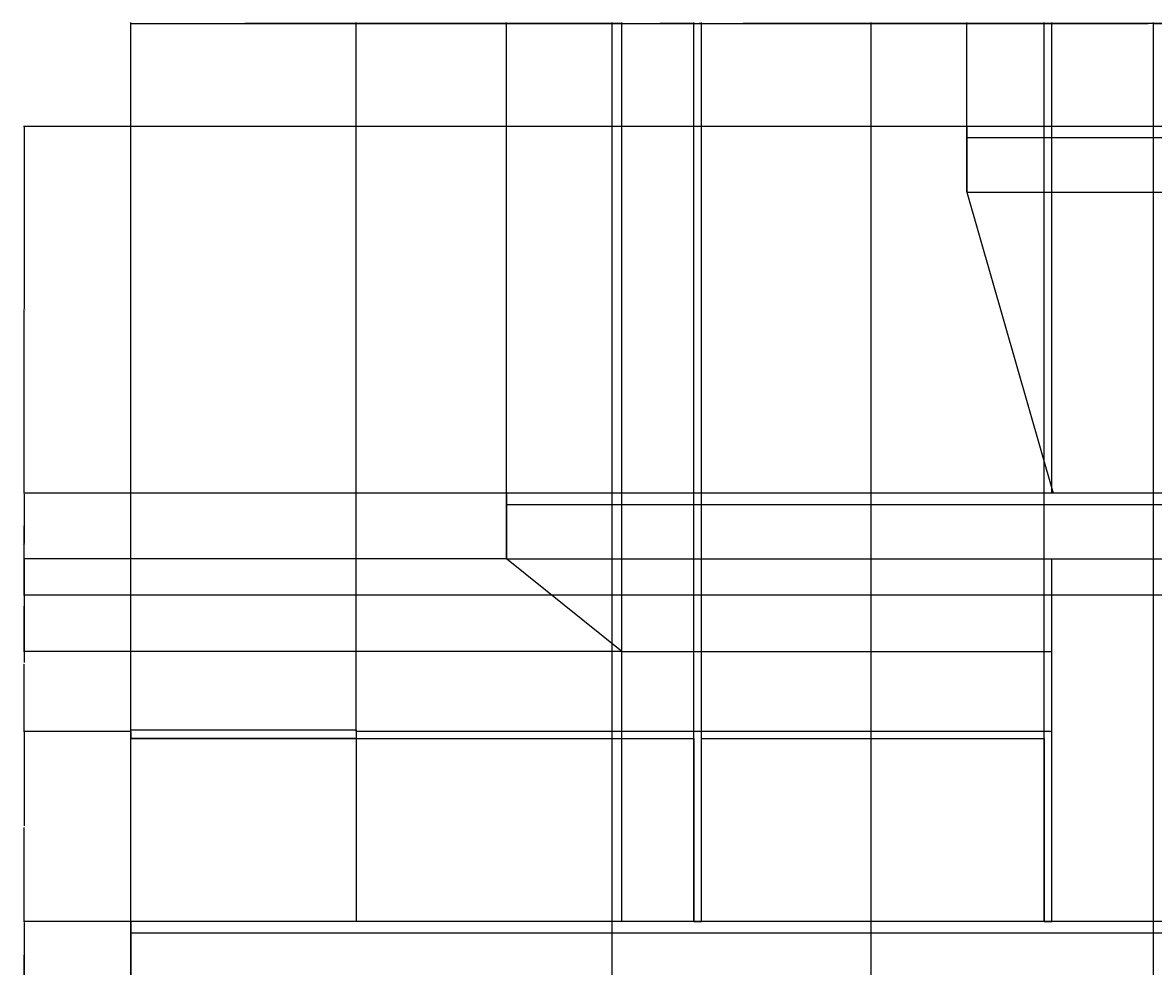
# Model space of a CAD drawing. Units: feet. Extents: x 2926 to 4178, y 965 to 1469.
# Tile 8 of 9: x 3641 to 3913, y 1241 to 1469. Entities that reach past the tile are written whole.
import ezdxf

# ---------------------------------------------------------------- set-up
doc = ezdxf.new("R2010")
doc.units = ezdxf.units.FT
doc.layers.add('A-ANNO-DIMS', color=2, linetype='Continuous', lineweight=18)
doc.layers.add('A-ELEV', color=7, linetype='Continuous', lineweight=25)
doc.styles.get("Standard").update_dxf_attribs({"font": 'arial.ttf'})
doc.dimstyles.get("Standard").update_dxf_attribs({"dimtxt": 0.18, "dimasz": 0.18, "dimexe": 0.18, "dimexo": 0.0625, "dimgap": 0.09, "dimtad": 0, "dimtih": 1, "dimtoh": 1, "dimdec": 1, "dimzin": 0, "dimdsep": 46, "dimlunit": 3, "dimtxsty": 'Standard', "dimcen": 0.09, "dimadec": 0, "dimazin": 0, "dimtfac": 1, "dimtdec": 1, "dimtofl": 0, "dimtmove": 0, "dimatfit": 3, "dimfxl": 1, "dimtolj": 1, "dimtzin": 0, "dimarcsym": 0})

# ---------------------------------------------------------------- blocks, each defined once
blk = doc.blocks.new('*D74')
at = {"layer": 'A-ANNO-DIMS', "color": 0, "lineweight": -2, "transparency": 16777216}
for p, q in [((3667.11, 1298.4), (3667.11, 1468.62)), ((3667.29, 1468.44), (3909.8, 1468.44)), ((4153.1, 1468.44), (3910.59, 1468.44)), ((4153.28, 1443.71), (4153.28, 1468.62))]:
    blk.add_line(p, q, dxfattribs=at)
at = {"layer": 'A-ANNO-DIMS', "color": 0, "transparency": 16777216}
for points in [[(3667.29, 1468.47), (3667.29, 1468.41), (3667.11, 1468.44)], [(4153.1, 1468.47), (4153.1, 1468.41), (4153.28, 1468.44)]]:
    blk.add_solid(points, dxfattribs=at)
at = {"layer": 'Defpoints', "color": 0, "transparency": 16777216}
for p in [(4153.28, 1468.44), (4153.28, 1443.64), (3667.11, 1298.33)]:
    blk.add_point(p, dxfattribs=at)
at = {"layer": 'A-ANNO-DIMS', "color": 0, "transparency": 16777216, "insert": (3910.2, 1468.44), "char_height": 0.18, "attachment_point": 5}
blk.add_mtext('\\A1;486.2', dxfattribs=at)
blk = doc.blocks.new('*D81')
at = {"layer": 'A-ANNO-DIMS', "color": 0, "lineweight": -2, "transparency": 16777216}
for p, q in [((3667.05, 1252.14), (3641.28, 1252.14)), ((3641.46, 1251.96), (3641.46, 1235.86)), ((3641.46, 1219.4), (3641.46, 1235.5)), ((3913.29, 1219.22), (3641.28, 1219.22))]:
    blk.add_line(p, q, dxfattribs=at)
at = {"layer": 'A-ANNO-DIMS', "color": 0, "transparency": 16777216}
for points in [[(3641.43, 1251.96), (3641.49, 1251.96), (3641.46, 1252.14)], [(3641.43, 1219.4), (3641.49, 1219.4), (3641.46, 1219.22)]]:
    blk.add_solid(points, dxfattribs=at)
at = {"layer": 'Defpoints', "color": 0, "transparency": 16777216}
for p in [(3641.46, 1252.14), (3667.11, 1252.14), (3913.35, 1219.22)]:
    blk.add_point(p, dxfattribs=at)
at = {"layer": 'A-ANNO-DIMS', "color": 0, "transparency": 16777216, "insert": (3641.46, 1235.68), "char_height": 0.18, "attachment_point": 5}
blk.add_mtext('\\A1;32.92', dxfattribs=at)
blk = doc.blocks.new('*D82')
at = {"layer": 'A-ANNO-DIMS', "color": 0, "lineweight": -2, "transparency": 16777216}
for p, q in [((3667.05, 1297.9), (3641.28, 1297.9)), ((3641.46, 1297.72), (3641.46, 1275.2)), ((3641.46, 1252.32), (3641.46, 1274.84)), ((3667.05, 1252.14), (3641.28, 1252.14))]:
    blk.add_line(p, q, dxfattribs=at)
at = {"layer": 'A-ANNO-DIMS', "color": 0, "transparency": 16777216}
for points in [[(3641.43, 1297.72), (3641.49, 1297.72), (3641.46, 1297.9)], [(3641.43, 1252.32), (3641.49, 1252.32), (3641.46, 1252.14)]]:
    blk.add_solid(points, dxfattribs=at)
at = {"layer": 'Defpoints', "color": 0, "transparency": 16777216}
for p in [(3641.46, 1297.9), (3667.11, 1297.9), (3667.11, 1252.14)]:
    blk.add_point(p, dxfattribs=at)
at = {"layer": 'A-ANNO-DIMS', "color": 0, "transparency": 16777216, "insert": (3641.46, 1275.02), "char_height": 0.18, "attachment_point": 5}
blk.add_mtext('\\A1;45.76', dxfattribs=at)
blk = doc.blocks.new('*D83')
at = {"layer": 'A-ANNO-DIMS', "color": 0, "lineweight": -2, "transparency": 16777216}
for p, q in [((4050.56, 1330.74), (3641.28, 1330.74)), ((3641.46, 1330.56), (3641.46, 1314.5)), ((3641.46, 1298.08), (3641.46, 1314.14)), ((3667.05, 1297.9), (3641.28, 1297.9))]:
    blk.add_line(p, q, dxfattribs=at)
at = {"layer": 'A-ANNO-DIMS', "color": 0, "transparency": 16777216}
for points in [[(3641.43, 1330.56), (3641.49, 1330.56), (3641.46, 1330.74)], [(3641.43, 1298.08), (3641.49, 1298.08), (3641.46, 1297.9)]]:
    blk.add_solid(points, dxfattribs=at)
at = {"layer": 'Defpoints', "color": 0, "transparency": 16777216}
for p in [(3641.46, 1330.74), (4050.62, 1330.74), (3667.11, 1297.9)]:
    blk.add_point(p, dxfattribs=at)
at = {"layer": 'A-ANNO-DIMS', "color": 0, "transparency": 16777216, "insert": (3641.46, 1314.32), "char_height": 0.18, "attachment_point": 5}
blk.add_mtext('\\A1;32.85', dxfattribs=at)
blk = doc.blocks.new('*D84')
at = {"layer": 'A-ANNO-DIMS', "color": 0, "lineweight": -2, "transparency": 16777216}
for p, q in [((3757.57, 1355.28), (3641.28, 1355.28)), ((3641.46, 1355.1), (3641.46, 1343.19)), ((3641.46, 1330.92), (3641.46, 1342.83)), ((4050.56, 1330.74), (3641.28, 1330.74))]:
    blk.add_line(p, q, dxfattribs=at)
at = {"layer": 'A-ANNO-DIMS', "color": 0, "transparency": 16777216}
for points in [[(3641.43, 1355.1), (3641.49, 1355.1), (3641.46, 1355.28)], [(3641.43, 1330.92), (3641.49, 1330.92), (3641.46, 1330.74)]]:
    blk.add_solid(points, dxfattribs=at)
at = {"layer": 'Defpoints', "color": 0, "transparency": 16777216}
for p in [(3641.46, 1355.28), (3757.63, 1355.28), (4050.62, 1330.74)]:
    blk.add_point(p, dxfattribs=at)
at = {"layer": 'A-ANNO-DIMS', "color": 0, "transparency": 16777216, "insert": (3641.46, 1343.01), "char_height": 0.18, "attachment_point": 5}
blk.add_mtext('\\A1;24.533', dxfattribs=at)
blk = doc.blocks.new('*D85')
at = {"layer": 'A-ANNO-DIMS', "color": 0, "lineweight": -2, "transparency": 16777216}
for p, q in [((3868.34, 1443.64), (3641.28, 1443.64)), ((3641.46, 1443.46), (3641.46, 1399.64)), ((3641.46, 1355.46), (3641.46, 1399.28)), ((3757.57, 1355.28), (3641.28, 1355.28))]:
    blk.add_line(p, q, dxfattribs=at)
at = {"layer": 'A-ANNO-DIMS', "color": 0, "transparency": 16777216}
for points in [[(3641.43, 1443.46), (3641.49, 1443.46), (3641.46, 1443.64)], [(3641.43, 1355.46), (3641.49, 1355.46), (3641.46, 1355.28)]]:
    blk.add_solid(points, dxfattribs=at)
at = {"layer": 'Defpoints', "color": 0, "transparency": 16777216}
for p in [(3641.46, 1443.64), (3868.41, 1443.64), (3757.63, 1355.28)]:
    blk.add_point(p, dxfattribs=at)
at = {"layer": 'A-ANNO-DIMS', "color": 0, "transparency": 16777216, "insert": (3641.46, 1399.46), "char_height": 0.18, "attachment_point": 5}
blk.add_mtext('\\A1;88.37', dxfattribs=at)
blk = doc.blocks.new('*D86')
at = {"layer": 'A-ANNO-DIMS', "color": 0, "lineweight": -2, "transparency": 16777216}
for p, q in [((3667.11, 1056.38), (3667.11, 1468.62)), ((3667.29, 1468.44), (3724.68, 1468.44)), ((3782.84, 1468.44), (3725.45, 1468.44)), ((3783.02, 1050.05), (3783.02, 1468.62))]:
    blk.add_line(p, q, dxfattribs=at)
at = {"layer": 'A-ANNO-DIMS', "color": 0, "transparency": 16777216}
for points in [[(3667.29, 1468.47), (3667.29, 1468.41), (3667.11, 1468.44)], [(3782.84, 1468.47), (3782.84, 1468.41), (3783.02, 1468.44)]]:
    blk.add_solid(points, dxfattribs=at)
at = {"layer": 'Defpoints', "color": 0, "transparency": 16777216}
for p in [(3783.02, 1468.44), (3667.11, 1056.32), (3783.02, 1049.98)]:
    blk.add_point(p, dxfattribs=at)
at = {"layer": 'A-ANNO-DIMS', "color": 0, "transparency": 16777216, "insert": (3725.07, 1468.44), "char_height": 0.18, "attachment_point": 5}
blk.add_mtext('\\A1;115.9', dxfattribs=at)
blk = doc.blocks.new('*D87')
at = {"layer": 'A-ANNO-DIMS', "color": 0, "lineweight": -2, "transparency": 16777216}
for p, q in [((3783.02, 1050.05), (3783.02, 1468.62)), ((3783.2, 1468.44), (3813.82, 1468.44)), ((3845.22, 1468.44), (3814.61, 1468.44)), ((3845.4, 1050.05), (3845.4, 1468.62))]:
    blk.add_line(p, q, dxfattribs=at)
at = {"layer": 'A-ANNO-DIMS', "color": 0, "transparency": 16777216}
for points in [[(3783.2, 1468.47), (3783.2, 1468.41), (3783.02, 1468.44)], [(3845.22, 1468.47), (3845.22, 1468.41), (3845.4, 1468.44)]]:
    blk.add_solid(points, dxfattribs=at)
at = {"layer": 'Defpoints', "color": 0, "transparency": 16777216}
for p in [(3845.4, 1468.44), (3783.02, 1049.98), (3845.4, 1049.98)]:
    blk.add_point(p, dxfattribs=at)
at = {"layer": 'A-ANNO-DIMS', "color": 0, "transparency": 16777216, "insert": (3814.21, 1468.44), "char_height": 0.18, "attachment_point": 5}
blk.add_mtext('\\A1;62.38', dxfattribs=at)
blk = doc.blocks.new('*D88')
at = {"layer": 'A-ANNO-DIMS', "color": 0, "lineweight": -2, "transparency": 16777216}
for p, q in [((3845.4, 1050.05), (3845.4, 1468.62)), ((3845.58, 1468.44), (3878.98, 1468.44)), ((3913.17, 1468.44), (3879.77, 1468.44)), ((3913.35, 1133.35), (3913.35, 1468.62))]:
    blk.add_line(p, q, dxfattribs=at)
at = {"layer": 'A-ANNO-DIMS', "color": 0, "transparency": 16777216}
for points in [[(3845.58, 1468.47), (3845.58, 1468.41), (3845.4, 1468.44)], [(3913.17, 1468.47), (3913.17, 1468.41), (3913.35, 1468.44)]]:
    blk.add_solid(points, dxfattribs=at)
at = {"layer": 'Defpoints', "color": 0, "transparency": 16777216}
for p in [(3913.35, 1468.44), (3913.35, 1133.29), (3845.4, 1049.98)]:
    blk.add_point(p, dxfattribs=at)
at = {"layer": 'A-ANNO-DIMS', "color": 0, "transparency": 16777216, "insert": (3879.38, 1468.44), "char_height": 0.18, "attachment_point": 5}
blk.add_mtext('\\A1;67.95', dxfattribs=at)
blk = doc.blocks.new('*D89')
at = {"layer": 'A-ANNO-DIMS', "color": 0, "lineweight": -2, "transparency": 16777216}
for p, q in [((3913.35, 1133.35), (3913.35, 1468.62)), ((3913.53, 1468.44), (3936.04, 1468.44)), ((3959.35, 1468.44), (3936.84, 1468.44)), ((3959.53, 1133.35), (3959.53, 1468.62))]:
    blk.add_line(p, q, dxfattribs=at)
at = {"layer": 'A-ANNO-DIMS', "color": 0, "transparency": 16777216}
for points in [[(3913.53, 1468.47), (3913.53, 1468.41), (3913.35, 1468.44)], [(3959.35, 1468.47), (3959.35, 1468.41), (3959.53, 1468.44)]]:
    blk.add_solid(points, dxfattribs=at)
at = {"layer": 'Defpoints', "color": 0, "transparency": 16777216}
for p in [(3959.53, 1468.44), (3913.35, 1133.29), (3959.53, 1133.29)]:
    blk.add_point(p, dxfattribs=at)
at = {"layer": 'A-ANNO-DIMS', "color": 0, "transparency": 16777216, "insert": (3936.44, 1468.44), "char_height": 0.18, "attachment_point": 5}
blk.add_mtext('\\A1;46.18', dxfattribs=at)
blk = doc.blocks.new('*D93')
at = {"layer": 'A-ANNO-DIMS', "color": 0, "lineweight": -2, "transparency": 16777216}
for p, q in [((3667.11, 1298.4), (3667.11, 1468.62)), ((3667.29, 1468.44), (3711.98, 1468.44)), ((3757.45, 1468.44), (3712.76, 1468.44)), ((3757.63, 1355.34), (3757.63, 1468.62))]:
    blk.add_line(p, q, dxfattribs=at)
at = {"layer": 'A-ANNO-DIMS', "color": 0, "transparency": 16777216}
for points in [[(3667.29, 1468.47), (3667.29, 1468.41), (3667.11, 1468.44)], [(3757.45, 1468.47), (3757.45, 1468.41), (3757.63, 1468.44)]]:
    blk.add_solid(points, dxfattribs=at)
at = {"layer": 'Defpoints', "color": 0, "transparency": 16777216}
for p in [(3757.63, 1468.44), (3757.63, 1355.28), (3667.11, 1298.33)]:
    blk.add_point(p, dxfattribs=at)
at = {"layer": 'A-ANNO-DIMS', "color": 0, "transparency": 16777216, "insert": (3712.37, 1468.44), "char_height": 0.18, "attachment_point": 5}
blk.add_mtext('\\A1;90.52', dxfattribs=at)
blk = doc.blocks.new('*D94')
at = {"layer": 'A-ANNO-DIMS', "color": 0, "lineweight": -2, "transparency": 16777216}
for p, q in [((3757.63, 1339.53), (3757.63, 1468.62)), ((3757.81, 1468.44), (3771.12, 1468.44)), ((3785.21, 1468.44), (3771.91, 1468.44)), ((3785.39, 1317.25), (3785.39, 1468.62))]:
    blk.add_line(p, q, dxfattribs=at)
at = {"layer": 'A-ANNO-DIMS', "color": 0, "transparency": 16777216}
for points in [[(3757.81, 1468.47), (3757.81, 1468.41), (3757.63, 1468.44)], [(3785.21, 1468.47), (3785.21, 1468.41), (3785.39, 1468.44)]]:
    blk.add_solid(points, dxfattribs=at)
at = {"layer": 'Defpoints', "color": 0, "transparency": 16777216}
for p in [(3785.39, 1468.44), (3757.63, 1339.46), (3785.39, 1317.18)]:
    blk.add_point(p, dxfattribs=at)
at = {"layer": 'A-ANNO-DIMS', "color": 0, "transparency": 16777216, "insert": (3771.51, 1468.44), "char_height": 0.18, "attachment_point": 5}
blk.add_mtext('\\A1;27.76', dxfattribs=at)
blk = doc.blocks.new('*D95')
at = {"layer": 'A-ANNO-DIMS', "color": 0, "lineweight": -2, "transparency": 16777216}
for p, q in [((3785.39, 1317.25), (3785.39, 1468.62)), ((3785.57, 1468.44), (3826.52, 1468.44)), ((3868.23, 1468.44), (3827.27, 1468.44)), ((3868.41, 1427.89), (3868.41, 1468.62))]:
    blk.add_line(p, q, dxfattribs=at)
at = {"layer": 'A-ANNO-DIMS', "color": 0, "transparency": 16777216}
for points in [[(3785.57, 1468.47), (3785.57, 1468.41), (3785.39, 1468.44)], [(3868.23, 1468.47), (3868.23, 1468.41), (3868.41, 1468.44)]]:
    blk.add_solid(points, dxfattribs=at)
at = {"layer": 'Defpoints', "color": 0, "transparency": 16777216}
for p in [(3868.41, 1468.44), (3868.41, 1427.83), (3785.39, 1317.18)]:
    blk.add_point(p, dxfattribs=at)
at = {"layer": 'A-ANNO-DIMS', "color": 0, "transparency": 16777216, "insert": (3826.9, 1468.44), "char_height": 0.18, "attachment_point": 5}
blk.add_mtext('\\A1;83.01', dxfattribs=at)
blk = doc.blocks.new('*D96')
at = {"layer": 'A-ANNO-DIMS', "color": 0, "lineweight": -2, "transparency": 16777216}
for p, q in [((3868.41, 1427.89), (3868.41, 1468.62)), ((3868.59, 1468.44), (3878.27, 1468.44)), ((3888.75, 1468.44), (3879.06, 1468.44)), ((3888.93, 1355.34), (3888.93, 1468.62))]:
    blk.add_line(p, q, dxfattribs=at)
at = {"layer": 'A-ANNO-DIMS', "color": 0, "transparency": 16777216}
for points in [[(3868.59, 1468.47), (3868.59, 1468.41), (3868.41, 1468.44)], [(3888.75, 1468.47), (3888.75, 1468.41), (3888.93, 1468.44)]]:
    blk.add_solid(points, dxfattribs=at)
at = {"layer": 'Defpoints', "color": 0, "transparency": 16777216}
for p in [(3888.93, 1468.44), (3868.41, 1427.83), (3888.93, 1355.28)]:
    blk.add_point(p, dxfattribs=at)
at = {"layer": 'A-ANNO-DIMS', "color": 0, "transparency": 16777216, "insert": (3878.67, 1468.44), "char_height": 0.18, "attachment_point": 5}
blk.add_mtext('\\A1;20.52', dxfattribs=at)
blk = doc.blocks.new('*D97')
at = {"layer": 'A-ANNO-DIMS', "color": 0, "lineweight": -2, "transparency": 16777216}
for p, q in [((3888.93, 1355.34), (3888.93, 1468.62)), ((3889.11, 1468.44), (3912.1, 1468.44)), ((3935.88, 1468.44), (3912.89, 1468.44)), ((3936.06, 1364.46), (3936.06, 1468.62))]:
    blk.add_line(p, q, dxfattribs=at)
at = {"layer": 'A-ANNO-DIMS', "color": 0, "transparency": 16777216}
for points in [[(3889.11, 1468.47), (3889.11, 1468.41), (3888.93, 1468.44)], [(3935.88, 1468.47), (3935.88, 1468.41), (3936.06, 1468.44)]]:
    blk.add_solid(points, dxfattribs=at)
at = {"layer": 'Defpoints', "color": 0, "transparency": 16777216}
for p in [(3936.06, 1468.44), (3936.06, 1364.4), (3888.93, 1355.28)]:
    blk.add_point(p, dxfattribs=at)
at = {"layer": 'A-ANNO-DIMS', "color": 0, "transparency": 16777216, "insert": (3912.49, 1468.44), "char_height": 0.18, "attachment_point": 5}
blk.add_mtext('\\A1;47.13', dxfattribs=at)
blk = doc.blocks.new('*D105')
at = {"layer": 'A-ANNO-DIMS', "color": 0, "lineweight": -2, "transparency": 16777216}
for p, q in [((3757.57, 1355.28), (3641.28, 1355.28)), ((3641.46, 1355.1), (3641.46, 1347.55)), ((3641.46, 1339.64), (3641.46, 1347.19)), ((3757.57, 1339.46), (3641.28, 1339.46))]:
    blk.add_line(p, q, dxfattribs=at)
at = {"layer": 'A-ANNO-DIMS', "color": 0, "transparency": 16777216}
for points in [[(3641.43, 1355.1), (3641.49, 1355.1), (3641.46, 1355.28)], [(3641.43, 1339.64), (3641.49, 1339.64), (3641.46, 1339.46)]]:
    blk.add_solid(points, dxfattribs=at)
at = {"layer": 'Defpoints', "color": 0, "transparency": 16777216}
for p in [(3641.46, 1355.28), (3757.63, 1355.28), (3757.63, 1339.46)]:
    blk.add_point(p, dxfattribs=at)
at = {"layer": 'A-ANNO-DIMS', "color": 0, "transparency": 16777216, "insert": (3641.46, 1347.37), "char_height": 0.18, "attachment_point": 5}
blk.add_mtext('\\A1;15.814', dxfattribs=at)
blk = doc.blocks.new('*D106')
at = {"layer": 'A-ANNO-DIMS', "color": 0, "lineweight": -2, "transparency": 16777216}
for p, q in [((3757.57, 1339.46), (3641.28, 1339.46)), ((3641.46, 1339.28), (3641.46, 1328.51)), ((3641.46, 1317.36), (3641.46, 1328.14)), ((3785.33, 1317.18), (3641.28, 1317.18))]:
    blk.add_line(p, q, dxfattribs=at)
at = {"layer": 'A-ANNO-DIMS', "color": 0, "transparency": 16777216}
for points in [[(3641.43, 1339.28), (3641.49, 1339.28), (3641.46, 1339.46)], [(3641.43, 1317.36), (3641.49, 1317.36), (3641.46, 1317.18)]]:
    blk.add_solid(points, dxfattribs=at)
at = {"layer": 'Defpoints', "color": 0, "transparency": 16777216}
for p in [(3641.46, 1339.46), (3757.63, 1339.46), (3785.39, 1317.18)]:
    blk.add_point(p, dxfattribs=at)
at = {"layer": 'A-ANNO-DIMS', "color": 0, "transparency": 16777216, "insert": (3641.46, 1328.32), "char_height": 0.18, "attachment_point": 5}
blk.add_mtext('\\A1;22.28', dxfattribs=at)
blk = doc.blocks.new('*D109')
at = {"layer": 'A-ANNO-DIMS', "color": 0, "lineweight": -2, "transparency": 16777216}
for p, q in [((3667.11, 1298.4), (3667.11, 1468.62)), ((3667.29, 1468.44), (3693.84, 1468.44)), ((3721.18, 1468.44), (3694.63, 1468.44)), ((3721.36, 1298.4), (3721.36, 1468.62))]:
    blk.add_line(p, q, dxfattribs=at)
at = {"layer": 'A-ANNO-DIMS', "color": 0, "transparency": 16777216}
for points in [[(3667.29, 1468.47), (3667.29, 1468.41), (3667.11, 1468.44)], [(3721.18, 1468.47), (3721.18, 1468.41), (3721.36, 1468.44)]]:
    blk.add_solid(points, dxfattribs=at)
at = {"layer": 'Defpoints', "color": 0, "transparency": 16777216}
for p in [(3721.36, 1468.44), (3667.11, 1298.33), (3721.36, 1298.33)]:
    blk.add_point(p, dxfattribs=at)
at = {"layer": 'A-ANNO-DIMS', "color": 0, "transparency": 16777216, "insert": (3694.24, 1468.44), "char_height": 0.18, "attachment_point": 5}
blk.add_mtext('\\A1;54.25', dxfattribs=at)
blk = doc.blocks.new('*D110')
at = {"layer": 'A-ANNO-DIMS', "color": 0, "lineweight": -2, "transparency": 16777216}
for p, q in [((3721.36, 1297.96), (3721.36, 1468.62)), ((3721.54, 1468.44), (3752.98, 1468.44)), ((3785.21, 1468.44), (3753.77, 1468.44)), ((3785.39, 1297.96), (3785.39, 1468.62))]:
    blk.add_line(p, q, dxfattribs=at)
at = {"layer": 'A-ANNO-DIMS', "color": 0, "transparency": 16777216}
for points in [[(3721.54, 1468.47), (3721.54, 1468.41), (3721.36, 1468.44)], [(3785.21, 1468.47), (3785.21, 1468.41), (3785.39, 1468.44)]]:
    blk.add_solid(points, dxfattribs=at)
at = {"layer": 'Defpoints', "color": 0, "transparency": 16777216}
for p in [(3785.39, 1468.44), (3721.36, 1297.9), (3785.39, 1297.9)]:
    blk.add_point(p, dxfattribs=at)
at = {"layer": 'A-ANNO-DIMS', "color": 0, "transparency": 16777216, "insert": (3753.38, 1468.44), "char_height": 0.18, "attachment_point": 5}
blk.add_mtext('\\A1;64.03', dxfattribs=at)
blk = doc.blocks.new('*D111')
at = {"layer": 'A-ANNO-DIMS', "color": 0, "lineweight": -2, "transparency": 16777216}
for p, q in [((3785.39, 1252.2), (3785.39, 1468.62)), ((3785.57, 1468.44), (3793.59, 1468.44)), ((3802.53, 1468.44), (3794.5, 1468.44)), ((3802.71, 1252.2), (3802.71, 1468.62))]:
    blk.add_line(p, q, dxfattribs=at)
at = {"layer": 'A-ANNO-DIMS', "color": 0, "transparency": 16777216}
for points in [[(3785.57, 1468.47), (3785.57, 1468.41), (3785.39, 1468.44)], [(3802.53, 1468.47), (3802.53, 1468.41), (3802.71, 1468.44)]]:
    blk.add_solid(points, dxfattribs=at)
at = {"layer": 'Defpoints', "color": 0, "transparency": 16777216}
for p in [(3802.71, 1468.44), (3785.39, 1252.14), (3802.71, 1252.14)]:
    blk.add_point(p, dxfattribs=at)
at = {"layer": 'A-ANNO-DIMS', "color": 0, "transparency": 16777216, "insert": (3794.05, 1468.44), "char_height": 0.18, "attachment_point": 5}
blk.add_mtext('\\A1;17.316', dxfattribs=at)
blk = doc.blocks.new('*D112')
at = {"layer": 'A-ANNO-DIMS', "color": 0, "lineweight": -2, "transparency": 16777216}
for p, q in [((3802.71, 1252.2), (3802.71, 1468.62)), ((3802.89, 1468.44), (3803.33, 1468.44)), ((3804.4, 1468.44), (3803.96, 1468.44)), ((3804.58, 1252.2), (3804.58, 1468.62))]:
    blk.add_line(p, q, dxfattribs=at)
at = {"layer": 'A-ANNO-DIMS', "color": 0, "transparency": 16777216}
for points in [[(3802.89, 1468.47), (3802.89, 1468.41), (3802.71, 1468.44)], [(3804.4, 1468.47), (3804.4, 1468.41), (3804.58, 1468.44)]]:
    blk.add_solid(points, dxfattribs=at)
at = {"layer": 'Defpoints', "color": 0, "transparency": 16777216}
for p in [(3804.58, 1468.44), (3802.71, 1252.14), (3804.58, 1252.14)]:
    blk.add_point(p, dxfattribs=at)
at = {"layer": 'A-ANNO-DIMS', "color": 0, "transparency": 16777216, "insert": (3803.64, 1468.44), "char_height": 0.18, "attachment_point": 5}
blk.add_mtext('\\A1;1.87', dxfattribs=at)
blk = doc.blocks.new('*D113')
at = {"layer": 'A-ANNO-DIMS', "color": 0, "lineweight": -2, "transparency": 16777216}
for p, q in [((3804.58, 1252.2), (3804.58, 1468.62)), ((3804.76, 1468.44), (3845.42, 1468.44)), ((3886.88, 1468.44), (3846.21, 1468.44)), ((3887.06, 1252.2), (3887.06, 1468.62))]:
    blk.add_line(p, q, dxfattribs=at)
at = {"layer": 'A-ANNO-DIMS', "color": 0, "transparency": 16777216}
for points in [[(3804.76, 1468.47), (3804.76, 1468.41), (3804.58, 1468.44)], [(3886.88, 1468.47), (3886.88, 1468.41), (3887.06, 1468.44)]]:
    blk.add_solid(points, dxfattribs=at)
at = {"layer": 'Defpoints', "color": 0, "transparency": 16777216}
for p in [(3887.06, 1468.44), (3804.58, 1252.14), (3887.06, 1252.14)]:
    blk.add_point(p, dxfattribs=at)
at = {"layer": 'A-ANNO-DIMS', "color": 0, "transparency": 16777216, "insert": (3845.82, 1468.44), "char_height": 0.18, "attachment_point": 5}
blk.add_mtext('\\A1;82.48', dxfattribs=at)
blk = doc.blocks.new('*D125')
at = {"layer": 'A-ANNO-DIMS', "color": 0, "lineweight": -2, "transparency": 16777216}
for p, q in [((3667.05, 1252.14), (3641.28, 1252.14)), ((3641.46, 1251.96), (3641.46, 1244.41)), ((3641.46, 1236.5), (3641.46, 1244.05)), ((3667.05, 1236.32), (3641.28, 1236.32))]:
    blk.add_line(p, q, dxfattribs=at)
at = {"layer": 'A-ANNO-DIMS', "color": 0, "transparency": 16777216}
for points in [[(3641.43, 1251.96), (3641.49, 1251.96), (3641.46, 1252.14)], [(3641.43, 1236.5), (3641.49, 1236.5), (3641.46, 1236.32)]]:
    blk.add_solid(points, dxfattribs=at)
at = {"layer": 'Defpoints', "color": 0, "transparency": 16777216}
for p in [(3641.46, 1252.14), (3667.11, 1252.14), (3667.11, 1236.32)]:
    blk.add_point(p, dxfattribs=at)
at = {"layer": 'A-ANNO-DIMS', "color": 0, "transparency": 16777216, "insert": (3641.46, 1244.23), "char_height": 0.18, "attachment_point": 5}
blk.add_mtext('\\A1;15.814', dxfattribs=at)

msp = doc.modelspace()

# ---------------------------------------------------------------- linework, layer by layer
at = {"layer": 'A-ELEV'}
for p, q in [((3868.4052, 1440.9727), (4153.2808, 1440.9727)), ((3868.4052, 1427.8302), (3889.2602, 1355.2778)), ((3888.9271, 1355.2778), (3888.9271, 1427.8302)), ((3757.63, 1352.606), (4094.6412, 1352.606)), ((3785.391, 1317.1829), (3757.63, 1339.4635)), ((3757.63, 1339.4635), (3888.9271, 1339.4635)), ((3888.9271, 1252.1389), (3888.9271, 1339.4635)), ((3785.391, 1317.1829), (3888.9271, 1317.1829)), ((3785.391, 1297.8963), (3785.391, 1317.1829)), ((3667.1119, 1236.3246), (3667.1119, 1298.3338)), ((3785.391, 1252.1389), (3785.391, 1296.2176)), ((3667.1119, 1249.4671), (4004.1232, 1249.4671))]:
    msp.add_line(p, q, dxfattribs=at)
for points in [[(4153.2808, 1443.6445), (3868.4052, 1443.6445), (3868.4052, 1427.8302), (4153.2808, 1427.8302)], [(4094.6412, 990.3246), (4094.6412, 1355.2778), (3757.63, 1355.2778), (3757.63, 1339.4635), (4078.8269, 1339.4635)], [(3667.1119, 1297.8963), (3667.1119, 1296.2176), (3802.7075, 1296.2176)], [(3888.9271, 1296.2176), (3888.9271, 1297.8963), (3721.3591, 1297.8963)], [(3802.7075, 1296.2176), (3802.7075, 1252.1389), (3804.5757, 1252.1389), (3804.5757, 1296.2176)], [(3804.5757, 1296.2176), (3887.0589, 1296.2176)], [(3887.0589, 1296.2176), (3887.0589, 1252.1389), (3888.9271, 1252.1389), (3888.9271, 1297.8963), (3887.0589, 1297.8963)], [(4004.1232, 1236.3246), (4004.1232, 1252.1389), (3667.1119, 1252.1389), (3667.1119, 1236.3246), (3988.3089, 1236.3246)]]:
    msp.add_lwpolyline(points, dxfattribs=at)
for points in [[(3721.3591, 1296.2176), (3667.1119, 1296.2176), (3667.1119, 1298.3338), (3721.3591, 1298.3338)], [(3667.1119, 1296.2176), (3721.3591, 1296.2176), (3721.3591, 1252.1389), (3667.1119, 1252.1389)]]:
    msp.add_lwpolyline(points, close=True, dxfattribs=at)

# ---------------------------------------------------------------- dimensions: what is measured, and where the dimension line sits
at = {"layer": 'A-ANNO-DIMS'}
for base, p1, p2, override, picture, middle in [((4153.2808, 1468.4445), (3667.1119, 1298.3338), (4153.2808, 1443.6445), {"dimdec": 1, "dimlfac": 1, "dimrnd": 0, "dimzin": 0, "dimdsep": 46, "dimlunit": 2}, '*D74', (3910.1964, 1468.4445)), ((3783.0229, 1468.4445), (3667.1119, 1056.3197), (3783.0229, 1049.9841), {"dimdec": 1, "dimlfac": 1, "dimrnd": 0, "dimzin": 0, "dimdsep": 46, "dimlunit": 2}, '*D86', (3725.0674, 1468.4445)), ((3757.63, 1468.4445), (3667.1119, 1298.3338), (3757.63, 1355.2778), {"dimdec": 2, "dimlfac": 1, "dimrnd": 0, "dimzin": 0, "dimdsep": 46, "dimlunit": 2}, '*D93', (3712.371, 1468.4445)), ((3721.3591, 1468.4445), (3667.1119, 1298.3338), (3721.3591, 1298.3338), {"dimdec": 2, "dimlfac": 1, "dimrnd": 0, "dimzin": 0, "dimdsep": 46, "dimlunit": 2}, '*D109', (3694.2355, 1468.4445)), ((3785.391, 1468.4445), (3721.3591, 1297.8963), (3785.391, 1297.8963), {"dimdec": 2, "dimlfac": 1, "dimrnd": 0, "dimzin": 0, "dimdsep": 46, "dimlunit": 2}, '*D110', (3753.3751, 1468.4445)), ((3785.391, 1468.4445), (3757.63, 1339.4635), (3785.391, 1317.1829), {"dimdec": 2, "dimlfac": 1, "dimrnd": 0, "dimzin": 0, "dimdsep": 46, "dimlunit": 2}, '*D94', (3771.5105, 1468.4445)), ((3845.3987, 1468.4445), (3783.0229, 1049.9841), (3845.3987, 1049.9841), {"dimdec": 2, "dimlfac": 1, "dimrnd": 0, "dimzin": 0, "dimdsep": 46, "dimlunit": 2}, '*D87', (3814.2108, 1468.4445)), ((3868.4052, 1468.4445), (3785.391, 1317.1829), (3868.4052, 1427.8302), {"dimdec": 2, "dimlfac": 1, "dimrnd": 0, "dimzin": 0, "dimdsep": 46, "dimlunit": 2}, '*D95', (3826.8981, 1468.4445)), ((3802.7075, 1468.44451), (3785.39104, 1252.13886), (3802.7075, 1252.13886), {"dimdec": 3, "dimlfac": 1, "dimrnd": 0, "dimzin": 0, "dimdsep": 46, "dimlunit": 2}, '*D111', (3794.04927, 1468.44451)), ((3804.5757, 1468.4445), (3802.7075, 1252.1389), (3804.5757, 1252.1389), {"dimdec": 2, "dimlfac": 1, "dimrnd": 0, "dimzin": 0, "dimdsep": 46, "dimlunit": 2}, '*D112', (3803.6416, 1468.4445)), ((3887.0589, 1468.4445), (3804.5757, 1252.1389), (3887.0589, 1252.1389), {"dimdec": 2, "dimlfac": 1, "dimrnd": 0, "dimzin": 0, "dimdsep": 46, "dimlunit": 2}, '*D113', (3845.8173, 1468.4445)), ((3913.3516, 1468.4445), (3845.3987, 1049.9841), (3913.3516, 1133.2879), {"dimdec": 2, "dimlfac": 1, "dimrnd": 0, "dimzin": 0, "dimdsep": 46, "dimlunit": 2}, '*D88', (3879.3752, 1468.4445)), ((3888.9271, 1468.4445), (3868.4052, 1427.8302), (3888.9271, 1355.2778), {"dimdec": 2, "dimlfac": 1, "dimrnd": 0, "dimzin": 0, "dimdsep": 46, "dimlunit": 2}, '*D96', (3878.6662, 1468.4445)), ((3936.0598, 1468.4445), (3888.9271, 1355.2778), (3936.0598, 1364.3965), {"dimdec": 2, "dimlfac": 1, "dimrnd": 0, "dimzin": 0, "dimdsep": 46, "dimlunit": 2}, '*D97', (3912.4935, 1468.4445)), ((3959.5291, 1468.4445), (3913.3516, 1133.2879), (3959.5291, 1133.2879), {"dimdec": 2, "dimlfac": 1, "dimrnd": 0, "dimzin": 0, "dimdsep": 46, "dimlunit": 2}, '*D89', (3936.4404, 1468.4445))]:
    dim = msp.add_linear_dim(base=base, p1=p1, p2=p2, dimstyle='Standard', override=override, dxfattribs=at)
    dim.commit()
    dim.dimension.update_dxf_attribs({"geometry": picture, "text_midpoint": middle})
for base, p1, p2, override, picture, middle in [((3641.4599, 1443.6445), (3757.63, 1355.2778), (3868.4052, 1443.6445), {"dimdec": 2, "dimlfac": 1, "dimrnd": 0, "dimzin": 0, "dimdsep": 46, "dimlunit": 2}, '*D85', (3641.4599, 1399.4612)), ((3641.4599, 1355.2778), (4050.6244, 1330.7444), (3757.63, 1355.2778), {"dimdec": 3, "dimlfac": 1, "dimrnd": 0, "dimzin": 0, "dimdsep": 46, "dimlunit": 2}, '*D84', (3641.4599, 1343.0111)), ((3641.4599, 1355.2778), (3757.63, 1339.4635), (3757.63, 1355.2778), {"dimdec": 3, "dimlfac": 1, "dimrnd": 0, "dimzin": 0, "dimdsep": 46, "dimlunit": 2}, '*D105', (3641.4599, 1347.3707)), ((3641.4599, 1339.4635), (3785.391, 1317.1829), (3757.63, 1339.4635), {"dimdec": 2, "dimlfac": 1, "dimrnd": 0, "dimzin": 0, "dimdsep": 46, "dimlunit": 2}, '*D106', (3641.4599, 1328.3232)), ((3641.4599, 1330.7444), (3667.1119, 1297.8963), (4050.6244, 1330.7444), {"dimdec": 2, "dimlfac": 1, "dimrnd": 0, "dimzin": 0, "dimdsep": 46, "dimlunit": 2}, '*D83', (3641.4599, 1314.3203)), ((3641.4599, 1297.8963), (3667.1119, 1252.1389), (3667.1119, 1297.8963), {"dimdec": 2, "dimlfac": 1, "dimrnd": 0, "dimzin": 0, "dimdsep": 46, "dimlunit": 2}, '*D82', (3641.4599, 1275.0176)), ((3641.4599, 1252.1389), (3667.1119, 1236.3246), (3667.1119, 1252.1389), {"dimdec": 3, "dimlfac": 1, "dimrnd": 0, "dimzin": 0, "dimdsep": 46, "dimlunit": 2}, '*D125', (3641.4599, 1244.2317)), ((3641.4599, 1252.1389), (3913.3516, 1219.2195), (3667.1119, 1252.1389), {"dimdec": 2, "dimlfac": 1, "dimrnd": 0, "dimzin": 0, "dimdsep": 46, "dimlunit": 2}, '*D81', (3641.4599, 1235.6792))]:
    dim = msp.add_linear_dim(base=base, p1=p1, p2=p2, angle=90, dimstyle='Standard', override=override, dxfattribs=at)
    dim.commit()
    dim.dimension.update_dxf_attribs({"geometry": picture, "text_midpoint": middle})

doc.saveas('drawing.dxf')
